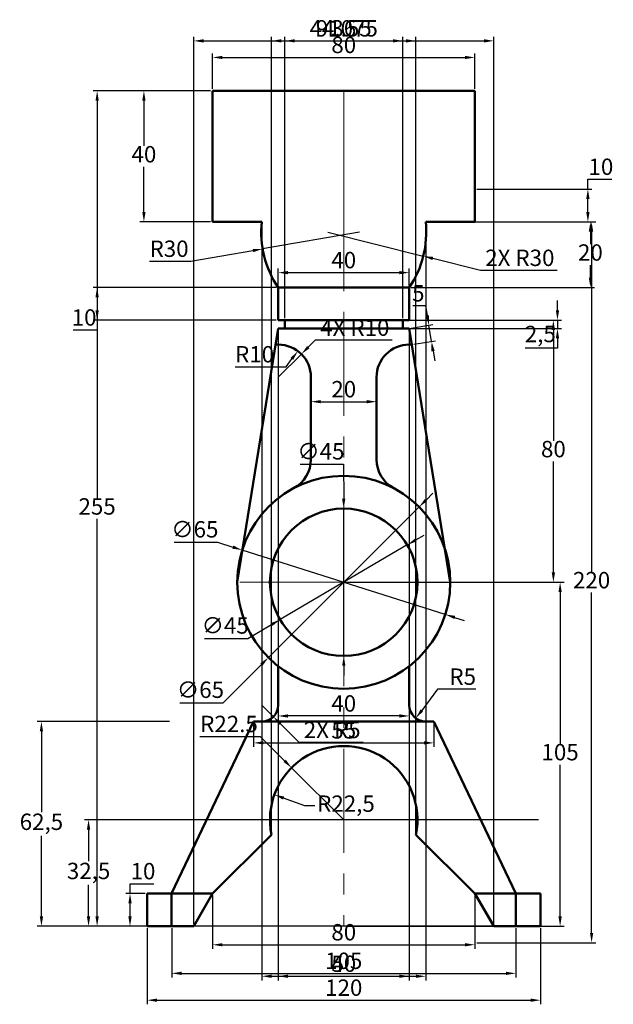
# Model space of a CAD drawing. Units: millimetres. Extents: x 61 to 242, y -47 to 253.
import ezdxf

# ---------------------------------------------------------------- set-up
doc = ezdxf.new("R2010")
doc.units = ezdxf.units.MM
doc.linetypes.add('CENTER', pattern=[50.8, 31.75, -6.35, 6.35, -6.35])
for name, color, linetype, lineweight in [('M-CNTR', 1, 'CENTER', 18), ('M-DIMS', 2, 'Continuous', 25), ('M-OUTL', 7, 'Continuous', 50)]:
    doc.layers.add(name, color=color, linetype=linetype, lineweight=lineweight)
doc.styles.get("Standard").update_dxf_attribs({"font": 'arial.ttf'})
doc.dimstyles.new('ISO-25', dxfattribs={"dimtxt": 5, "dimasz": 3, "dimexe": 1.25, "dimexo": 0.625, "dimtad": 1, "dimtih": 1, "dimtoh": 1, "dimtxsty": 'Standard', "dimcen": 2.5, "dimadec": 0, "dimazin": 0, "dimtfac": 1, "dimtmove": 0, "dimatfit": 3, "dimfxl": 1, "dimarcsym": 0})

# ---------------------------------------------------------------- blocks, each defined once
blk = doc.blocks.new('*D1')
at = {"layer": 'Defpoints', "color": 0, "transparency": 16777216}
for p in [(120.12, 231.51), (99.15, 191.51), (120.12, 191.51)]:
    blk.add_point(p, dxfattribs=at)
at = {"layer": 'M-DIMS', "color": 0, "lineweight": -2, "transparency": 16777216}
for p, q in [((119.49, 231.51), (97.9, 231.51)), ((99.15, 228.51), (99.15, 214.69)), ((99.15, 194.51), (99.15, 208.34)), ((119.49, 191.51), (97.9, 191.51))]:
    blk.add_line(p, q, dxfattribs=at)
at = {"layer": 'M-DIMS', "color": 0, "transparency": 16777216}
for points in [[(98.65, 228.51), (99.65, 228.51), (99.15, 231.51)], [(98.65, 194.51), (99.65, 194.51), (99.15, 191.51)]]:
    blk.add_solid(points, dxfattribs=at)
at = {"layer": 'M-DIMS', "color": 0, "transparency": 16777216, "insert": (99.15, 211.51), "char_height": 5, "attachment_point": 5}
blk.add_mtext('40', dxfattribs=at)
blk = doc.blocks.new('*D2')
at = {"layer": 'Defpoints', "color": 0, "transparency": 16777216}
for p in [(200.12, 241.7), (120.12, 231.51), (200.12, 231.51)]:
    blk.add_point(p, dxfattribs=at)
at = {"layer": 'M-DIMS', "color": 0, "lineweight": -2, "transparency": 16777216}
for p, q in [((120.12, 232.14), (120.12, 242.95)), ((123.12, 241.7), (197.12, 241.7)), ((200.12, 232.14), (200.12, 242.95))]:
    blk.add_line(p, q, dxfattribs=at)
at = {"layer": 'M-DIMS', "color": 0, "transparency": 16777216}
for points in [[(123.12, 242.2), (123.12, 241.2), (120.12, 241.7)], [(197.12, 242.2), (197.12, 241.2), (200.12, 241.7)]]:
    blk.add_solid(points, dxfattribs=at)
at = {"layer": 'M-DIMS', "color": 0, "transparency": 16777216, "insert": (160.12, 244.88), "char_height": 5, "attachment_point": 5}
blk.add_mtext('80', dxfattribs=at)
blk = doc.blocks.new('*D3')
at = {"layer": 'Defpoints', "color": 0, "transparency": 16777216}
for p in [(200.12, 201.51), (234.61, 201.51), (200.12, 191.51)]:
    blk.add_point(p, dxfattribs=at)
at = {"layer": 'M-DIMS', "color": 0, "lineweight": -2, "transparency": 16777216}
for p, q in [((234.61, 201.51), (234.61, 204.51)), ((234.61, 204.51), (241.91, 204.51)), ((200.74, 201.51), (235.86, 201.51)), ((234.61, 194.51), (234.61, 198.51)), ((200.74, 191.51), (235.86, 191.51))]:
    blk.add_line(p, q, dxfattribs=at)
at = {"layer": 'M-DIMS', "color": 0, "transparency": 16777216}
for points in [[(234.11, 198.51), (235.11, 198.51), (234.61, 201.51)], [(234.11, 194.51), (235.11, 194.51), (234.61, 191.51)]]:
    blk.add_solid(points, dxfattribs=at)
at = {"layer": 'M-DIMS', "color": 0, "transparency": 16777216, "insert": (238.58, 207.69), "char_height": 5, "attachment_point": 5}
blk.add_mtext('10', dxfattribs=at)
blk = doc.blocks.new('*D4')
at = {"layer": 'Defpoints', "color": 0, "transparency": 16777216}
for p in [(180.12, 176.02), (140.12, 171.51), (180.12, 171.51)]:
    blk.add_point(p, dxfattribs=at)
at = {"layer": 'M-DIMS', "color": 0, "lineweight": -2, "transparency": 16777216}
for p, q in [((140.12, 172.14), (140.12, 177.27)), ((143.12, 176.02), (177.12, 176.02)), ((180.12, 172.14), (180.12, 177.27))]:
    blk.add_line(p, q, dxfattribs=at)
at = {"layer": 'M-DIMS', "color": 0, "transparency": 16777216}
for points in [[(143.12, 176.52), (143.12, 175.52), (140.12, 176.02)], [(177.12, 176.52), (177.12, 175.52), (180.12, 176.02)]]:
    blk.add_solid(points, dxfattribs=at)
at = {"layer": 'M-DIMS', "color": 0, "transparency": 16777216, "insert": (160.12, 179.2), "char_height": 5, "attachment_point": 5}
blk.add_mtext('40', dxfattribs=at)
blk = doc.blocks.new('*D5')
at = {"layer": 'Defpoints', "color": 0, "transparency": 16777216}
for p in [(164.95, 188.35), (135.38, 183.27)]:
    blk.add_point(p, dxfattribs=at)
at = {"layer": 'M-DIMS', "color": 0, "lineweight": -2, "transparency": 16777216}
for p, q in [((164.95, 188.35), (135.38, 183.27)), ((113.42, 179.49), (132.42, 182.76)), ((100.86, 179.49), (113.42, 179.49))]:
    blk.add_line(p, q, dxfattribs=at)
at = {"layer": 'M-DIMS', "color": 0, "transparency": 16777216}
blk.add_solid([(132.34, 183.25), (132.51, 182.26), (135.38, 183.27)], dxfattribs=at)
at = {"layer": 'M-DIMS', "color": 0, "transparency": 16777216, "insert": (106.83, 182.67), "char_height": 5, "attachment_point": 5}
blk.add_mtext('R30', dxfattribs=at)
blk = doc.blocks.new('*D6')
at = {"layer": 'Defpoints', "color": 0, "transparency": 16777216}
for p in [(150.12, 144.08), (170.12, 144.08), (170.12, 136.63)]:
    blk.add_point(p, dxfattribs=at)
at = {"layer": 'M-DIMS', "color": 0, "lineweight": -2, "transparency": 16777216}
for p, q in [((150.12, 143.45), (150.12, 135.38)), ((170.12, 143.45), (170.12, 135.38)), ((153.12, 136.63), (167.12, 136.63))]:
    blk.add_line(p, q, dxfattribs=at)
at = {"layer": 'M-DIMS', "color": 0, "transparency": 16777216}
for points in [[(153.12, 137.13), (153.12, 136.13), (150.12, 136.63)], [(167.12, 137.13), (167.12, 136.13), (170.12, 136.63)]]:
    blk.add_solid(points, dxfattribs=at)
at = {"layer": 'M-DIMS', "color": 0, "transparency": 16777216, "insert": (160.12, 139.8), "char_height": 5, "attachment_point": 5}
blk.add_mtext('20', dxfattribs=at)
blk = doc.blocks.new('*D7')
at = {"layer": 'Defpoints', "color": 0, "transparency": 16777216}
for p in [(146.1, 152.09), (140.12, 144.08)]:
    blk.add_point(p, dxfattribs=at)
at = {"layer": 'M-DIMS', "color": 0, "lineweight": -2, "transparency": 16777216}
for p, q in [((126.96, 147.28), (142.51, 147.28)), ((142.51, 147.28), (144.31, 149.68))]:
    blk.add_line(p, q, dxfattribs=at)
at = {"layer": 'M-DIMS', "color": 0, "transparency": 16777216}
blk.add_solid([(143.91, 149.98), (144.71, 149.38), (146.1, 152.09)], dxfattribs=at)
at = {"layer": 'M-DIMS', "color": 0, "transparency": 16777216, "insert": (132.92, 150.46), "char_height": 5, "attachment_point": 5}
blk.add_mtext('R10', dxfattribs=at)
blk = doc.blocks.new('*D8')
at = {"layer": 'Defpoints', "color": 0, "transparency": 16777216}
for p in [(129.14, 91.34), (191.1, 71.69)]:
    blk.add_point(p, dxfattribs=at)
at = {"layer": 'M-DIMS', "color": 0, "lineweight": -2, "transparency": 16777216}
for p, q in [((108.37, 93.71), (121.64, 93.71)), ((121.64, 93.71), (126.28, 92.24)), ((191.1, 71.69), (129.14, 91.34)), ((193.96, 70.78), (196.81, 69.88))]:
    blk.add_line(p, q, dxfattribs=at)
at = {"layer": 'M-DIMS', "color": 0, "transparency": 16777216}
for points in [[(126.43, 92.72), (126.12, 91.77), (129.14, 91.34)], [(194.11, 71.26), (193.8, 70.31), (191.1, 71.69)]]:
    blk.add_solid(points, dxfattribs=at)
at = {"layer": 'M-DIMS', "color": 0, "transparency": 16777216, "insert": (114.69, 97.03), "char_height": 5, "attachment_point": 5}
blk.add_mtext('∅65', dxfattribs=at)
blk = doc.blocks.new('*D9')
at = {"layer": 'Defpoints', "color": 0, "transparency": 16777216}
for p in [(179.52, 92.9), (140.71, 70.13)]:
    blk.add_point(p, dxfattribs=at)
at = {"layer": 'M-DIMS', "color": 0, "lineweight": -2, "transparency": 16777216}
for p, q in [((182.11, 94.42), (184.7, 95.93)), ((179.52, 92.9), (140.71, 70.13)), ((130.89, 64.37), (138.12, 68.61)), ((117.62, 64.37), (130.89, 64.37))]:
    blk.add_line(p, q, dxfattribs=at)
at = {"layer": 'M-DIMS', "color": 0, "transparency": 16777216}
for points in [[(181.86, 94.85), (182.36, 93.99), (179.52, 92.9)], [(137.87, 69.04), (138.37, 68.18), (140.71, 70.13)]]:
    blk.add_solid(points, dxfattribs=at)
at = {"layer": 'M-DIMS', "color": 0, "transparency": 16777216, "insert": (123.94, 67.68), "char_height": 5, "attachment_point": 5}
blk.add_mtext('∅45', dxfattribs=at)
blk = doc.blocks.new('*D10')
at = {"layer": 'Defpoints', "color": 0, "transparency": 16777216}
for p in [(138.96, 16.66), (160.12, 9.01)]:
    blk.add_point(p, dxfattribs=at)
at = {"layer": 'M-DIMS', "color": 0, "lineweight": -2, "transparency": 16777216}
for p, q in [((148.27, 13.3), (141.78, 15.64)), ((151.27, 13.3), (148.27, 13.3))]:
    blk.add_line(p, q, dxfattribs=at)
at = {"layer": 'M-DIMS', "color": 0, "transparency": 16777216}
blk.add_solid([(141.95, 16.11), (141.61, 15.17), (138.96, 16.66)], dxfattribs=at)
at = {"layer": 'M-DIMS', "color": 0, "transparency": 16777216, "insert": (160.8, 13.3), "char_height": 5, "attachment_point": 5}
blk.add_mtext('R22,5', dxfattribs=at)
blk = doc.blocks.new('*D11')
at = {"layer": 'Defpoints', "color": 0, "transparency": 16777216}
for p in [(185.12, 44.01), (182.13, 40)]:
    blk.add_point(p, dxfattribs=at)
at = {"layer": 'M-DIMS', "color": 0, "lineweight": -2, "transparency": 16777216}
for p, q in [((188.75, 48.9), (183.92, 42.41)), ((200.47, 48.9), (188.75, 48.9))]:
    blk.add_line(p, q, dxfattribs=at)
at = {"layer": 'M-DIMS', "color": 0, "transparency": 16777216}
blk.add_solid([(183.52, 42.71), (184.32, 42.11), (182.13, 40)], dxfattribs=at)
at = {"layer": 'M-DIMS', "color": 0, "transparency": 16777216, "insert": (196.42, 52.06), "char_height": 5, "attachment_point": 5}
blk.add_mtext('R5', dxfattribs=at)
blk = doc.blocks.new('*D12')
at = {"layer": 'Defpoints', "color": 0, "transparency": 16777216}
for p in [(132.62, 39.01), (187.62, 39.01), (187.62, 32.49)]:
    blk.add_point(p, dxfattribs=at)
at = {"layer": 'M-DIMS', "color": 0, "lineweight": -2, "transparency": 16777216}
for p, q in [((132.62, 38.39), (132.62, 31.24)), ((187.62, 38.39), (187.62, 31.24)), ((135.62, 32.49), (184.62, 32.49))]:
    blk.add_line(p, q, dxfattribs=at)
at = {"layer": 'M-DIMS', "color": 0, "transparency": 16777216}
for points in [[(135.62, 32.99), (135.62, 31.99), (132.62, 32.49)], [(184.62, 32.99), (184.62, 31.99), (187.62, 32.49)]]:
    blk.add_solid(points, dxfattribs=at)
at = {"layer": 'M-DIMS', "color": 0, "transparency": 16777216, "insert": (160.12, 35.66), "char_height": 5, "attachment_point": 5}
blk.add_mtext('55', dxfattribs=at)
blk = doc.blocks.new('*D13')
at = {"layer": 'Defpoints', "color": 0, "transparency": 16777216}
for p in [(140.12, 44.01), (180.12, 44.01), (140.12, 40.71)]:
    blk.add_point(p, dxfattribs=at)
at = {"layer": 'M-DIMS', "color": 0, "lineweight": -2, "transparency": 16777216}
for p, q in [((140.12, 43.39), (140.12, 39.46)), ((180.12, 43.39), (180.12, 39.46)), ((177.12, 40.71), (143.12, 40.71))]:
    blk.add_line(p, q, dxfattribs=at)
at = {"layer": 'M-DIMS', "color": 0, "transparency": 16777216}
for points in [[(143.12, 41.21), (143.12, 40.21), (140.12, 40.71)], [(177.12, 41.21), (177.12, 40.21), (180.12, 40.71)]]:
    blk.add_solid(points, dxfattribs=at)
at = {"layer": 'M-DIMS', "color": 0, "transparency": 16777216, "insert": (160.12, 43.88), "char_height": 5, "attachment_point": 5}
blk.add_mtext('40', dxfattribs=at)
blk = doc.blocks.new('*D14')
at = {"layer": 'Defpoints', "color": 0, "transparency": 16777216}
for p in [(160.12, 161.51), (224.08, 161.51), (160.12, 81.51)]:
    blk.add_point(p, dxfattribs=at)
at = {"layer": 'M-DIMS', "color": 0, "lineweight": -2, "transparency": 16777216}
for p, q in [((160.74, 161.51), (225.33, 161.51)), ((224.08, 158.51), (224.08, 124.69)), ((224.08, 84.51), (224.08, 118.34)), ((160.74, 81.51), (225.33, 81.51))]:
    blk.add_line(p, q, dxfattribs=at)
at = {"layer": 'M-DIMS', "color": 0, "transparency": 16777216}
for points in [[(223.58, 158.51), (224.58, 158.51), (224.08, 161.51)], [(223.58, 84.51), (224.58, 84.51), (224.08, 81.51)]]:
    blk.add_solid(points, dxfattribs=at)
at = {"layer": 'M-DIMS', "color": 0, "transparency": 16777216, "insert": (224.08, 121.51), "char_height": 5, "attachment_point": 5}
blk.add_mtext('80', dxfattribs=at)
blk = doc.blocks.new('*D15')
at = {"layer": 'Defpoints', "color": 0, "transparency": 16777216}
for p in [(178.12, 161.51), (178.12, 159.01), (225.33, 159.01)]:
    blk.add_point(p, dxfattribs=at)
at = {"layer": 'M-DIMS', "color": 0, "lineweight": -2, "transparency": 16777216}
for p, q in [((225.33, 164.51), (225.33, 167.51)), ((178.74, 161.51), (226.58, 161.51)), ((225.33, 161.51), (225.33, 159.01)), ((178.74, 159.01), (226.58, 159.01)), ((225.33, 156.01), (225.33, 153.01)), ((225.33, 153.01), (215.48, 153.01))]:
    blk.add_line(p, q, dxfattribs=at)
at = {"layer": 'M-DIMS', "color": 0, "transparency": 16777216}
for points in [[(224.83, 164.51), (225.83, 164.51), (225.33, 161.51)], [(224.83, 156.01), (225.83, 156.01), (225.33, 159.01)]]:
    blk.add_solid(points, dxfattribs=at)
at = {"layer": 'M-DIMS', "color": 0, "transparency": 16777216, "insert": (220.09, 156.64), "char_height": 5, "attachment_point": 5}
blk.add_mtext('2,5', dxfattribs=at)
blk = doc.blocks.new('*D16')
at = {"layer": 'Defpoints', "color": 0, "transparency": 16777216}
for p in [(186.1, 159.98), (180.12, 159.01), (180.91, 154.08)]:
    blk.add_point(p, dxfattribs=at)
at = {"layer": 'M-DIMS', "color": 0, "lineweight": -2, "transparency": 16777216}
for p, q in [((185.15, 165.9), (181.21, 165.9)), ((185.63, 162.94), (185.15, 165.9)), ((180.73, 159.11), (187.34, 160.18)), ((186.9, 155.04), (186.1, 159.98)), ((181.53, 154.18), (188.13, 155.24)), ((187.38, 152.08), (187.86, 149.12))]:
    blk.add_line(p, q, dxfattribs=at)
at = {"layer": 'M-DIMS', "color": 0, "transparency": 16777216}
for points in [[(186.12, 163.02), (185.13, 162.86), (186.1, 159.98)], [(187.87, 152.16), (186.88, 152), (186.9, 155.04)]]:
    blk.add_solid(points, dxfattribs=at)
at = {"layer": 'M-DIMS', "color": 0, "transparency": 16777216, "insert": (182.87, 169.07), "char_height": 5, "attachment_point": 5}
blk.add_mtext('5', dxfattribs=at)
blk = doc.blocks.new('*D17')
at = {"layer": 'Defpoints', "color": 0, "transparency": 16777216}
for p in [(94.91, -13.49), (100.12, -13.49), (100.12, -23.49)]:
    blk.add_point(p, dxfattribs=at)
at = {"layer": 'M-DIMS', "color": 0, "lineweight": -2, "transparency": 16777216}
for p, q in [((94.91, -13.49), (94.91, -10.49)), ((94.91, -10.49), (102.21, -10.49)), ((99.49, -13.49), (93.66, -13.49)), ((94.91, -20.49), (94.91, -16.49)), ((99.49, -23.49), (93.66, -23.49))]:
    blk.add_line(p, q, dxfattribs=at)
at = {"layer": 'M-DIMS', "color": 0, "transparency": 16777216}
for points in [[(94.41, -16.49), (95.41, -16.49), (94.91, -13.49)], [(94.41, -20.49), (95.41, -20.49), (94.91, -23.49)]]:
    blk.add_solid(points, dxfattribs=at)
at = {"layer": 'M-DIMS', "color": 0, "transparency": 16777216, "insert": (98.87, -7.31), "char_height": 5, "attachment_point": 5}
blk.add_mtext('10', dxfattribs=at)
blk = doc.blocks.new('*D18')
at = {"layer": 'Defpoints', "color": 0, "transparency": 16777216}
for p in [(120.12, -13.49), (200.12, -13.49), (200.12, -29.13)]:
    blk.add_point(p, dxfattribs=at)
at = {"layer": 'M-DIMS', "color": 0, "lineweight": -2, "transparency": 16777216}
for p, q in [((120.12, -14.11), (120.12, -30.38)), ((200.12, -14.11), (200.12, -30.38)), ((123.12, -29.13), (197.12, -29.13))]:
    blk.add_line(p, q, dxfattribs=at)
at = {"layer": 'M-DIMS', "color": 0, "transparency": 16777216}
for points in [[(123.12, -28.63), (123.12, -29.63), (120.12, -29.13)], [(197.12, -28.63), (197.12, -29.63), (200.12, -29.13)]]:
    blk.add_solid(points, dxfattribs=at)
at = {"layer": 'M-DIMS', "color": 0, "transparency": 16777216, "insert": (160.12, -25.95), "char_height": 5, "attachment_point": 5}
blk.add_mtext('80', dxfattribs=at)
blk = doc.blocks.new('*D19')
at = {"layer": 'Defpoints', "color": 0, "transparency": 16777216}
for p in [(107.62, -23.49), (212.62, -23.49), (212.62, -37.85)]:
    blk.add_point(p, dxfattribs=at)
at = {"layer": 'M-DIMS', "color": 0, "lineweight": -2, "transparency": 16777216}
for p, q in [((107.62, -24.11), (107.62, -39.1)), ((212.62, -24.11), (212.62, -39.1)), ((110.62, -37.85), (209.62, -37.85))]:
    blk.add_line(p, q, dxfattribs=at)
at = {"layer": 'M-DIMS', "color": 0, "transparency": 16777216}
for points in [[(110.62, -37.35), (110.62, -38.35), (107.62, -37.85)], [(209.62, -37.35), (209.62, -38.35), (212.62, -37.85)]]:
    blk.add_solid(points, dxfattribs=at)
at = {"layer": 'M-DIMS', "color": 0, "transparency": 16777216, "insert": (160.12, -34.67), "char_height": 5, "attachment_point": 5}
blk.add_mtext('105', dxfattribs=at)
blk = doc.blocks.new('*D20')
at = {"layer": 'Defpoints', "color": 0, "transparency": 16777216}
for p in [(100.12, -23.49), (220.12, -23.49), (220.12, -46.05)]:
    blk.add_point(p, dxfattribs=at)
at = {"layer": 'M-DIMS', "color": 0, "lineweight": -2, "transparency": 16777216}
for p, q in [((100.12, -24.11), (100.12, -47.3)), ((220.12, -24.11), (220.12, -47.3)), ((103.12, -46.05), (217.12, -46.05))]:
    blk.add_line(p, q, dxfattribs=at)
at = {"layer": 'M-DIMS', "color": 0, "transparency": 16777216}
for points in [[(103.12, -45.55), (103.12, -46.55), (100.12, -46.05)], [(217.12, -45.55), (217.12, -46.55), (220.12, -46.05)]]:
    blk.add_solid(points, dxfattribs=at)
at = {"layer": 'M-DIMS', "color": 0, "transparency": 16777216, "insert": (160.12, -42.87), "char_height": 5, "attachment_point": 5}
blk.add_mtext('120', dxfattribs=at)
blk = doc.blocks.new('*D21')
at = {"layer": 'Defpoints', "color": 0, "transparency": 16777216}
for p in [(200.12, 191.51), (200.12, -28.49), (235.74, -28.49)]:
    blk.add_point(p, dxfattribs=at)
at = {"layer": 'M-DIMS', "color": 0, "lineweight": -2, "transparency": 16777216}
for p, q in [((200.74, 191.51), (236.99, 191.51)), ((235.74, 188.51), (235.74, 84.69)), ((235.74, -25.49), (235.74, 78.34)), ((200.74, -28.49), (236.99, -28.49))]:
    blk.add_line(p, q, dxfattribs=at)
at = {"layer": 'M-DIMS', "color": 0, "transparency": 16777216}
for points in [[(235.24, 188.51), (236.24, 188.51), (235.74, 191.51)], [(235.24, -25.49), (236.24, -25.49), (235.74, -28.49)]]:
    blk.add_solid(points, dxfattribs=at)
at = {"layer": 'M-DIMS', "color": 0, "transparency": 16777216, "insert": (235.74, 81.51), "char_height": 5, "attachment_point": 5}
blk.add_mtext('220', dxfattribs=at)
blk = doc.blocks.new('*D22')
at = {"layer": 'Defpoints', "color": 0, "transparency": 16777216}
for p in [(160.12, 81.51), (160.12, -23.49), (226.13, -23.49)]:
    blk.add_point(p, dxfattribs=at)
at = {"layer": 'M-DIMS', "color": 0, "lineweight": -2, "transparency": 16777216}
for p, q in [((160.74, 81.51), (227.38, 81.51)), ((226.13, 78.51), (226.13, 32.19)), ((226.13, -20.49), (226.13, 25.84)), ((160.74, -23.49), (227.38, -23.49))]:
    blk.add_line(p, q, dxfattribs=at)
at = {"layer": 'M-DIMS', "color": 0, "transparency": 16777216}
for points in [[(225.63, 78.51), (226.63, 78.51), (226.13, 81.51)], [(225.63, -20.49), (226.63, -20.49), (226.13, -23.49)]]:
    blk.add_solid(points, dxfattribs=at)
at = {"layer": 'M-DIMS', "color": 0, "transparency": 16777216, "insert": (226.13, 29.01), "char_height": 5, "attachment_point": 5}
blk.add_mtext('105', dxfattribs=at)
blk = doc.blocks.new('*D23')
at = {"layer": 'Defpoints', "color": 0, "transparency": 16777216}
for p in [(82.26, 9.01), (220.12, 9.01), (220.12, -23.49)]:
    blk.add_point(p, dxfattribs=at)
at = {"layer": 'M-DIMS', "color": 0, "lineweight": -2, "transparency": 16777216}
for p, q in [((219.49, 9.01), (81.01, 9.01)), ((82.26, 6.01), (82.26, -3.61)), ((82.26, -20.49), (82.26, -10.87)), ((219.49, -23.49), (81.01, -23.49))]:
    blk.add_line(p, q, dxfattribs=at)
at = {"layer": 'M-DIMS', "color": 0, "transparency": 16777216}
for points in [[(81.76, 6.01), (82.76, 6.01), (82.26, 9.01)], [(81.76, -20.49), (82.76, -20.49), (82.26, -23.49)]]:
    blk.add_solid(points, dxfattribs=at)
at = {"layer": 'M-DIMS', "color": 0, "transparency": 16777216, "insert": (82.26, -7.24), "char_height": 5, "attachment_point": 5}
blk.add_mtext('32,5', dxfattribs=at)
blk = doc.blocks.new('*D24')
at = {"layer": 'Defpoints', "color": 0, "transparency": 16777216}
for p in [(67.88, 39.01), (107.62, 39.01), (107.62, -23.49)]:
    blk.add_point(p, dxfattribs=at)
at = {"layer": 'M-DIMS', "color": 0, "lineweight": -2, "transparency": 16777216}
for p, q in [((106.99, 39.01), (66.63, 39.01)), ((67.88, 36.01), (67.88, 11.39)), ((67.88, -20.49), (67.88, 4.13)), ((106.99, -23.49), (66.63, -23.49))]:
    blk.add_line(p, q, dxfattribs=at)
at = {"layer": 'M-DIMS', "color": 0, "transparency": 16777216}
for points in [[(67.38, 36.01), (68.38, 36.01), (67.88, 39.01)], [(67.38, -20.49), (68.38, -20.49), (67.88, -23.49)]]:
    blk.add_solid(points, dxfattribs=at)
at = {"layer": 'M-DIMS', "color": 0, "transparency": 16777216, "insert": (67.88, 7.76), "char_height": 5, "attachment_point": 5}
blk.add_mtext('62,5', dxfattribs=at)
blk = doc.blocks.new('*D25')
at = {"layer": 'Defpoints', "color": 0, "transparency": 16777216}
for p in [(84.87, 231.51), (120.12, 231.51), (100.12, -23.49)]:
    blk.add_point(p, dxfattribs=at)
at = {"layer": 'M-DIMS', "color": 0, "lineweight": -2, "transparency": 16777216}
for p, q in [((119.49, 231.51), (83.62, 231.51)), ((84.87, 228.51), (84.87, 107.19)), ((84.87, -20.49), (84.87, 100.84)), ((99.49, -23.49), (83.62, -23.49))]:
    blk.add_line(p, q, dxfattribs=at)
at = {"layer": 'M-DIMS', "color": 0, "transparency": 16777216}
for points in [[(84.37, 228.51), (85.37, 228.51), (84.87, 231.51)], [(84.37, -20.49), (85.37, -20.49), (84.87, -23.49)]]:
    blk.add_solid(points, dxfattribs=at)
at = {"layer": 'M-DIMS', "color": 0, "transparency": 16777216, "insert": (84.87, 104.01), "char_height": 5, "attachment_point": 5}
blk.add_mtext('255', dxfattribs=at)
blk = doc.blocks.new('*D26')
at = {"layer": 'Defpoints', "color": 0, "transparency": 16777216}
for p in [(135.12, 191.51), (185.12, 191.51), (185.12, -38.74)]:
    blk.add_point(p, dxfattribs=at)
at = {"layer": 'M-DIMS', "color": 0, "lineweight": -2, "transparency": 16777216}
for p, q in [((135.12, 190.89), (135.12, -39.99)), ((185.12, 190.89), (185.12, -39.99)), ((138.12, -38.74), (182.12, -38.74))]:
    blk.add_line(p, q, dxfattribs=at)
at = {"layer": 'M-DIMS', "color": 0, "transparency": 16777216}
for points in [[(138.12, -38.24), (138.12, -39.24), (135.12, -38.74)], [(182.12, -38.24), (182.12, -39.24), (185.12, -38.74)]]:
    blk.add_solid(points, dxfattribs=at)
at = {"layer": 'M-DIMS', "color": 0, "transparency": 16777216, "insert": (160.12, -35.56), "char_height": 5, "attachment_point": 5}
blk.add_mtext('50', dxfattribs=at)
blk = doc.blocks.new('*D27')
at = {"layer": 'Defpoints', "color": 0, "transparency": 16777216}
for p in [(140.12, 171.51), (84.87, 161.51), (140.12, 161.51)]:
    blk.add_point(p, dxfattribs=at)
at = {"layer": 'M-DIMS', "color": 0, "lineweight": -2, "transparency": 16777216}
for p, q in [((139.49, 171.51), (83.62, 171.51)), ((84.87, 168.51), (84.87, 164.51)), ((139.49, 161.51), (83.62, 161.51)), ((84.87, 161.51), (84.87, 158.51)), ((84.87, 158.51), (77.57, 158.51))]:
    blk.add_line(p, q, dxfattribs=at)
at = {"layer": 'M-DIMS', "color": 0, "transparency": 16777216}
for points in [[(84.37, 168.51), (85.37, 168.51), (84.87, 171.51)], [(84.37, 164.51), (85.37, 164.51), (84.87, 161.51)]]:
    blk.add_solid(points, dxfattribs=at)
at = {"layer": 'M-DIMS', "color": 0, "transparency": 16777216, "insert": (80.9, 161.69), "char_height": 5, "attachment_point": 5}
blk.add_mtext('10', dxfattribs=at)
blk = doc.blocks.new('*D28')
at = {"layer": 'Defpoints', "color": 0, "transparency": 16777216}
for p in [(185.12, 191.51), (180.12, 171.51), (235.37, 171.51)]:
    blk.add_point(p, dxfattribs=at)
at = {"layer": 'M-DIMS', "color": 0, "lineweight": -2, "transparency": 16777216}
for p, q in [((185.74, 191.51), (236.62, 191.51)), ((235.37, 188.51), (235.37, 184.69)), ((235.37, 174.51), (235.37, 178.34)), ((180.74, 171.51), (236.62, 171.51))]:
    blk.add_line(p, q, dxfattribs=at)
at = {"layer": 'M-DIMS', "color": 0, "transparency": 16777216}
for points in [[(234.87, 188.51), (235.87, 188.51), (235.37, 191.51)], [(234.87, 174.51), (235.87, 174.51), (235.37, 171.51)]]:
    blk.add_solid(points, dxfattribs=at)
at = {"layer": 'M-DIMS', "color": 0, "transparency": 16777216, "insert": (235.37, 181.51), "char_height": 5, "attachment_point": 5}
blk.add_mtext('20', dxfattribs=at)
blk = doc.blocks.new('*D29')
at = {"layer": 'Defpoints', "color": 0, "transparency": 16777216}
for p in [(178.12, 246.76), (142.12, 161.51), (178.12, 161.51)]:
    blk.add_point(p, dxfattribs=at)
at = {"layer": 'M-DIMS', "color": 0, "lineweight": -2, "transparency": 16777216}
for p, q in [((142.12, 162.14), (142.12, 248.01)), ((145.12, 246.76), (175.12, 246.76)), ((178.12, 162.14), (178.12, 248.01))]:
    blk.add_line(p, q, dxfattribs=at)
at = {"layer": 'M-DIMS', "color": 0, "transparency": 16777216}
for points in [[(145.12, 247.26), (145.12, 246.26), (142.12, 246.76)], [(175.12, 247.26), (175.12, 246.26), (178.12, 246.76)]]:
    blk.add_solid(points, dxfattribs=at)
at = {"layer": 'M-DIMS', "color": 0, "transparency": 16777216, "insert": (160.12, 249.94), "char_height": 5, "attachment_point": 5}
blk.add_mtext('36', dxfattribs=at)
blk = doc.blocks.new('*D30')
at = {"layer": 'Defpoints', "color": 0, "transparency": 16777216}
for p in [(140.12, 159.01), (180.12, 159.01), (180.12, -38.74)]:
    blk.add_point(p, dxfattribs=at)
at = {"layer": 'M-DIMS', "color": 0, "lineweight": -2, "transparency": 16777216}
for p, q in [((140.12, 158.39), (140.12, -39.99)), ((180.12, 158.39), (180.12, -39.99)), ((143.12, -38.74), (177.12, -38.74))]:
    blk.add_line(p, q, dxfattribs=at)
at = {"layer": 'M-DIMS', "color": 0, "transparency": 16777216}
for points in [[(143.12, -38.24), (143.12, -39.24), (140.12, -38.74)], [(177.12, -38.24), (177.12, -39.24), (180.12, -38.74)]]:
    blk.add_solid(points, dxfattribs=at)
at = {"layer": 'M-DIMS', "color": 0, "transparency": 16777216, "insert": (160.12, -35.56), "char_height": 5, "attachment_point": 5}
blk.add_mtext('40', dxfattribs=at)
blk = doc.blocks.new('*D31')
at = {"layer": 'Defpoints', "color": 0, "transparency": 16777216}
for p in [(182.15, 246.76), (138.08, 4.48), (182.15, 4.48)]:
    blk.add_point(p, dxfattribs=at)
at = {"layer": 'M-DIMS', "color": 0, "lineweight": -2, "transparency": 16777216}
for p, q in [((138.08, 5.1), (138.08, 248.01)), ((141.08, 246.76), (179.15, 246.76)), ((182.15, 5.1), (182.15, 248.01))]:
    blk.add_line(p, q, dxfattribs=at)
at = {"layer": 'M-DIMS', "color": 0, "transparency": 16777216}
for points in [[(141.08, 247.26), (141.08, 246.26), (138.08, 246.76)], [(179.15, 247.26), (179.15, 246.26), (182.15, 246.76)]]:
    blk.add_solid(points, dxfattribs=at)
at = {"layer": 'M-DIMS', "color": 0, "transparency": 16777216, "insert": (160.12, 249.94), "char_height": 5, "attachment_point": 5}
blk.add_mtext('44.075', dxfattribs=at)
blk = doc.blocks.new('*D32')
at = {"layer": 'Defpoints', "color": 0, "transparency": 16777216}
for p in [(205.89, 246.76), (114.34, -23.49), (205.89, -23.49)]:
    blk.add_point(p, dxfattribs=at)
at = {"layer": 'M-DIMS', "color": 0, "lineweight": -2, "transparency": 16777216}
for p, q in [((114.34, -22.86), (114.34, 248.01)), ((117.34, 246.76), (202.89, 246.76)), ((205.89, -22.86), (205.89, 248.01))]:
    blk.add_line(p, q, dxfattribs=at)
at = {"layer": 'M-DIMS', "color": 0, "transparency": 16777216}
for points in [[(117.34, 247.26), (117.34, 246.26), (114.34, 246.76)], [(202.89, 247.26), (202.89, 246.26), (205.89, 246.76)]]:
    blk.add_solid(points, dxfattribs=at)
at = {"layer": 'M-DIMS', "color": 0, "transparency": 16777216, "insert": (160.12, 249.94), "char_height": 5, "attachment_point": 5}
blk.add_mtext('91.55', dxfattribs=at)
blk = doc.blocks.new('*D33')
at = {"layer": 'Defpoints', "color": 0, "transparency": 16777216}
for p in [(183.1, 104.49), (137.13, 58.53)]:
    blk.add_point(p, dxfattribs=at)
at = {"layer": 'M-DIMS', "color": 0, "lineweight": -2, "transparency": 16777216}
for p, q in [((185.22, 106.61), (187.34, 108.74)), ((183.1, 104.49), (137.13, 58.53)), ((123.34, 44.75), (135.01, 56.41)), ((110.08, 44.75), (123.34, 44.75))]:
    blk.add_line(p, q, dxfattribs=at)
at = {"layer": 'M-DIMS', "color": 0, "transparency": 16777216}
for points in [[(184.87, 106.97), (185.57, 106.26), (183.1, 104.49)], [(134.66, 56.77), (135.37, 56.06), (137.13, 58.53)]]:
    blk.add_solid(points, dxfattribs=at)
at = {"layer": 'M-DIMS', "color": 0, "transparency": 16777216, "insert": (116.4, 48.06), "char_height": 5, "attachment_point": 5}
blk.add_mtext('∅65', dxfattribs=at)
blk = doc.blocks.new('*D34')
at = {"layer": 'Defpoints', "color": 0, "transparency": 16777216}
for p in [(160.1, 104.01), (160.13, 59.01)]:
    blk.add_point(p, dxfattribs=at)
at = {"layer": 'M-DIMS', "color": 0, "lineweight": -2, "transparency": 16777216}
for p, q in [((146.83, 117.51), (160.09, 117.51)), ((160.09, 117.51), (160.1, 107.01)), ((160.13, 59.01), (160.1, 104.01)), ((160.13, 56.01), (160.13, 53.01))]:
    blk.add_line(p, q, dxfattribs=at)
at = {"layer": 'M-DIMS', "color": 0, "transparency": 16777216}
for points in [[(160.6, 107.01), (159.6, 107.01), (160.1, 104.01)], [(160.63, 56.01), (159.63, 56.01), (160.13, 59.01)]]:
    blk.add_solid(points, dxfattribs=at)
at = {"layer": 'M-DIMS', "color": 0, "transparency": 16777216, "insert": (153.15, 120.83), "char_height": 5, "attachment_point": 5}
blk.add_mtext('∅45', dxfattribs=at)
blk = doc.blocks.new('*D35')
at = {"layer": 'Defpoints', "color": 0, "transparency": 16777216}
for p in [(155.28, 188.35), (184.39, 181.07)]:
    blk.add_point(p, dxfattribs=at)
at = {"layer": 'M-DIMS', "color": 0, "lineweight": -2, "transparency": 16777216}
for p, q in [((155.28, 188.35), (184.39, 181.07)), ((201.85, 176.71), (187.3, 180.34)), ((225.23, 176.71), (201.85, 176.71))]:
    blk.add_line(p, q, dxfattribs=at)
at = {"layer": 'M-DIMS', "color": 0, "transparency": 16777216}
blk.add_solid([(187.42, 180.83), (187.18, 179.86), (184.39, 181.07)], dxfattribs=at)
at = {"layer": 'M-DIMS', "color": 0, "transparency": 16777216, "insert": (213.85, 179.89), "char_height": 5, "attachment_point": 5}
blk.add_mtext('2X R30', dxfattribs=at)
blk = doc.blocks.new('*D36')
at = {"layer": 'Defpoints', "color": 0, "transparency": 16777216}
for p in [(144.19, 24.91), (160.12, 9.01)]:
    blk.add_point(p, dxfattribs=at)
at = {"layer": 'M-DIMS', "color": 0, "lineweight": -2, "transparency": 16777216}
for p, q in [((116.2, 34.45), (134.64, 34.45)), ((134.64, 34.45), (142.07, 27.03)), ((160.12, 9.01), (144.19, 24.91))]:
    blk.add_line(p, q, dxfattribs=at)
at = {"layer": 'M-DIMS', "color": 0, "transparency": 16777216}
blk.add_solid([(142.42, 27.38), (141.71, 26.67), (144.19, 24.91)], dxfattribs=at)
at = {"layer": 'M-DIMS', "color": 0, "transparency": 16777216, "insert": (125.11, 37.62), "char_height": 5, "attachment_point": 5}
blk.add_mtext('R22.5', dxfattribs=at)
blk = doc.blocks.new('*D37')
at = {"layer": 'Defpoints', "color": 0, "transparency": 16777216}
for p in [(147.19, 151.15), (140.12, 144.08)]:
    blk.add_point(p, dxfattribs=at)
at = {"layer": 'M-DIMS', "color": 0, "lineweight": -2, "transparency": 16777216}
for p, q in [((151.43, 155.39), (149.31, 153.27)), ((174.93, 155.39), (151.43, 155.39)), ((140.12, 144.08), (147.19, 151.15))]:
    blk.add_line(p, q, dxfattribs=at)
at = {"layer": 'M-DIMS', "color": 0, "transparency": 16777216}
blk.add_solid([(148.95, 153.62), (149.66, 152.92), (147.19, 151.15)], dxfattribs=at)
at = {"layer": 'M-DIMS', "color": 0, "transparency": 16777216, "insert": (163.49, 158.57), "char_height": 5, "attachment_point": 5}
blk.add_mtext('4X R10', dxfattribs=at)
blk = doc.blocks.new('*D38')
at = {"layer": 'Defpoints', "color": 0, "transparency": 16777216}
for p in [(135.12, 44.01), (138.65, 40.48)]:
    blk.add_point(p, dxfattribs=at)
at = {"layer": 'M-DIMS', "color": 0, "lineweight": -2, "transparency": 16777216}
for p, q in [((135.12, 44.01), (138.65, 40.48)), ((146.5, 32.63), (140.77, 38.36)), ((166.06, 32.63), (146.5, 32.63))]:
    blk.add_line(p, q, dxfattribs=at)
at = {"layer": 'M-DIMS', "color": 0, "transparency": 16777216}
blk.add_solid([(141.13, 38.71), (140.42, 38), (138.65, 40.48)], dxfattribs=at)
at = {"layer": 'M-DIMS', "color": 0, "transparency": 16777216, "insert": (156.59, 35.8), "char_height": 5, "attachment_point": 5}
blk.add_mtext('2X R5', dxfattribs=at)

msp = doc.modelspace()

# ---------------------------------------------------------------- linework, layer by layer
at = {"layer": 'M-CNTR'}
for p, q in [((160.1154, 171.5135), (160.1154, 231.5135)), ((160.1154, 193.8867), (160.1154, 222.2813)), ((160.1154, 171.0055), (160.1154, 193.8867)), ((160.1154, 81.5135), (160.1154, 171.0055)), ((160.1154, 81.5135), (127.6154, 81.5135)), ((160.1154, 81.5135), (160.1154, 49.0135)), ((160.1154, 81.5135), (192.6154, 81.5135)), ((160.1154, 81.5135), (160.1154, -23.4865)), ((192.6154, 81.5135), (216.1928, 81.5135))]:
    msp.add_line(p, q, dxfattribs=at)
at = {"layer": 'M-OUTL'}
for p, q in [((160.1154, 231.5135), (120.1154, 231.5135)), ((120.1154, 231.5135), (120.1154, 191.5135)), ((160.1154, 231.5135), (200.1154, 231.5135)), ((200.1154, 231.5135), (200.1154, 191.5135)), ((120.1154, 191.5135), (135.1154, 191.5135)), ((200.1154, 191.5135), (185.1154, 191.5135)), ((140.1154, 161.5135), (140.1154, 171.5135)), ((140.1154, 171.5135), (180.1154, 171.5135)), ((180.1154, 171.5135), (180.1154, 161.5135)), ((160.1154, 161.5135), (140.1154, 161.5135)), ((142.1154, 161.5135), (142.1154, 159.0135)), ((160.1154, 161.5135), (180.1154, 161.5135)), ((178.1154, 161.5135), (178.1154, 159.0135)), ((140.1154, 159.0135), (127.6154, 81.5135)), ((140.1154, 159.0135), (180.1154, 159.0135)), ((180.1154, 159.0135), (192.6154, 81.5135)), ((180.1154, 159.0135), (180.9116, 154.0773)), ((140.1154, 154.0773), (139.3193, 154.0773)), ((180.9116, 154.0773), (180.1154, 154.0773)), ((150.1154, 144.0773), (150.1154, 119.0135)), ((170.1154, 144.0773), (170.1154, 119.0135)), ((140.1154, 49.0135), (140.1154, 55.8961)), ((180.1154, 44.0135), (180.1154, 55.8961)), ((140.1154, 49.0135), (140.1154, 44.0135)), ((132.6154, 39.0135), (107.6154, -13.4865)), ((135.1154, 39.0135), (132.6154, 39.0135)), ((135.1154, 39.0135), (185.1154, 39.0135)), ((185.1154, 39.0135), (187.6154, 39.0135)), ((187.6154, 39.0135), (212.6154, -13.4865)), ((120.1154, -13.4865), (138.0777, 4.4758)), ((200.1154, -13.4865), (182.1531, 4.4758)), ((100.1154, -23.4865), (100.1154, -13.4865)), ((100.1154, -13.4865), (120.1154, -13.4865)), ((107.6154, -23.4865), (107.6154, -13.4865)), ((120.1154, -13.4865), (114.3419, -23.4865)), ((200.1154, -13.4865), (205.8889, -23.4865)), ((200.1154, -13.4865), (220.1154, -13.4865)), ((212.6154, -23.4865), (212.6154, -13.4865)), ((212.6154, -23.4865), (212.6154, -13.4865)), ((220.1154, -13.4865), (220.1154, -23.4865)), ((114.3419, -23.4865), (100.1154, -23.4865)), ((114.3419, -23.4865), (107.6154, -23.4865)), ((205.8889, -23.4865), (220.1154, -23.4865)), ((205.8889, -23.4865), (212.6154, -23.4865))]:
    msp.add_line(p, q, dxfattribs=at)
for radius in [32.5, 22.5]:
    msp.add_circle((160.1154, 81.5135), radius, dxfattribs=at)
for centre, radius, start, end in [((164.9478, 188.3466), 30, 173.940365, 214.132122), ((155.283, 188.3466), 30, 325.867878, 6.059635), ((140.1154, 144.0773), 10, 0, 90), ((180.1154, 144.0773), 10, 90, 180), ((140.1154, 119.0135), 10, 298.072487, 0), ((180.1154, 119.0135), 10, 180, 241.927513), ((135.1154, 44.0135), 5, 270, 0), ((185.1154, 44.0135), 5, 180, 270), ((160.1154, 9.0135), 22.5, 348.365088, 191.634912)]:
    msp.add_arc(centre, radius, start, end, dxfattribs=at)

# ---------------------------------------------------------------- dimensions: what is measured, and where the dimension line sits
at = {"layer": 'M-DIMS'}
for base, p1, p2, override, picture, middle in [((205.8889, 246.7635), (114.3419, -23.4865), (205.8889, -23.4865), {"dimdec": 2, "dimlfac": 1, "dimrnd": 0, "dimzin": 0, "dimdsep": 46, "dimlunit": 2}, '*D32', (160.1154, 249.9414)), ((182.1531, 246.7635), (138.0777, 4.4758), (182.1531, 4.4758), {"dimdec": 3, "dimlfac": 1, "dimrnd": 0, "dimzin": 0, "dimdsep": 46, "dimlunit": 2}, '*D31', (160.1154, 249.9414)), ((178.1154, 246.7635), (142.1154, 161.5135), (178.1154, 161.5135), {"dimdec": 0, "dimlfac": 1, "dimrnd": 0, "dimzin": 0, "dimdsep": 46, "dimlunit": 2}, '*D29', (160.1154, 249.9431)), ((200.1154, 241.7028), (120.1154, 231.5135), (200.1154, 231.5135), {"dimclrd": 0, "dimclre": 0, "dimclrt": 0}, '*D2', (160.1154, 244.8807)), ((185.1154, -38.7365), (135.1154, 191.5135), (185.1154, 191.5135), {"dimdec": 0, "dimlfac": 1, "dimrnd": 0, "dimzin": 0, "dimdsep": 46, "dimlunit": 2}, '*D26', (160.1154, -35.5586)), ((180.1154, 176.0185), (140.1154, 171.5135), (180.1154, 171.5135), {"dimclrd": 0, "dimclre": 0, "dimclrt": 0}, '*D4', (160.1154, 179.1964)), ((180.1154, -38.7365), (140.1154, 159.0135), (180.1154, 159.0135), {"dimdec": 0, "dimlfac": 1, "dimrnd": 0, "dimzin": 0, "dimdsep": 46, "dimlunit": 2}, '*D30', (160.1154, -35.5586)), ((170.1154, 136.6268), (150.1154, 144.0773), (170.1154, 144.0773), {"dimclrd": 0, "dimclre": 0, "dimclrt": 0}, '*D6', (160.1154, 139.8047)), ((140.1154, 40.7053), (180.1154, 44.0135), (140.1154, 44.0135), {"dimclrd": 0, "dimclre": 0, "dimclrt": 0}, '*D13', (160.1154, 43.8832)), ((187.6154, 32.4943), (132.6154, 39.0135), (187.6154, 39.0135), {"dimclrd": 0, "dimclre": 0, "dimclrt": 0}, '*D12', (160.1154, 35.662)), ((200.1154, -29.132), (120.1154, -13.4865), (200.1154, -13.4865), {"dimclrd": 0, "dimclre": 0, "dimclrt": 0}, '*D18', (160.1154, -25.9541)), ((220.1154, -46.0522), (100.1154, -23.4865), (220.1154, -23.4865), {"dimclrd": 0, "dimclre": 0, "dimclrt": 0}, '*D20', (160.1154, -42.8743)), ((212.6154, -37.8499), (107.6154, -23.4865), (212.6154, -23.4865), {"dimclrd": 0, "dimclre": 0, "dimclrt": 0}, '*D19', (160.1154, -34.672))]:
    dim = msp.add_linear_dim(base=base, p1=p1, p2=p2, dimstyle='ISO-25', override=override, dxfattribs=at)
    dim.commit()
    dim.dimension.update_dxf_attribs({"geometry": picture, "text_midpoint": middle})
for base, p1, p2, override, picture, middle in [((84.8654, 231.5135), (100.1154, -23.4865), (120.1154, 231.5135), {"dimdec": 0, "dimlfac": 1, "dimrnd": 0, "dimzin": 0, "dimdsep": 46, "dimlunit": 2}, '*D25', (84.8654, 104.0135)), ((99.1453, 191.5135), (120.1154, 231.5135), (120.1154, 191.5135), {"dimclrd": 0, "dimclre": 0, "dimclrt": 0}, '*D1', (99.1453, 211.5135)), ((234.614, 201.5135), (200.1154, 191.5135), (200.1154, 201.5135), {"dimclrd": 0, "dimclre": 0, "dimclrt": 0}, '*D3', (238.5763, 207.6914)), ((235.3654, 171.5135), (185.1154, 191.5135), (180.1154, 171.5135), {"dimdec": 0, "dimlfac": 1, "dimrnd": 0, "dimzin": 0, "dimdsep": 46, "dimlunit": 2}, '*D28', (235.3654, 181.5135)), ((235.7375, -28.4865), (200.1154, 191.5135), (200.1154, -28.4865), {"dimclrd": 0, "dimclre": 0, "dimclrt": 0}, '*D21', (235.7375, 81.5135)), ((84.8654, 161.5135), (140.1154, 171.5135), (140.1154, 161.5135), {"dimdec": 0, "dimlfac": 1, "dimrnd": 0, "dimzin": 0, "dimdsep": 46, "dimlunit": 2}, '*D27', (80.9031, 161.6914)), ((225.3288, 159.0135), (178.1154, 161.5135), (178.1154, 159.0135), {"dimclrd": 0, "dimclre": 0, "dimclrt": 0}, '*D15', (220.091, 156.6433)), ((224.0788, 161.5135), (160.1154, 81.5135), (160.1154, 161.5135), {"dimclrd": 0, "dimclre": 0, "dimclrt": 0}, '*D14', (224.0788, 121.5135)), ((226.1293, -23.4865), (160.1154, 81.5135), (160.1154, -23.4865), {"dimclrd": 0, "dimclre": 0, "dimclrt": 0}, '*D22', (226.1293, 29.0135)), ((67.878, 39.0135), (107.6154, -23.4865), (107.6154, 39.0135), {"dimclrd": 0, "dimclre": 0, "dimclrt": 0}, '*D24', (67.878, 7.7635)), ((82.2623, 9.0135), (220.1154, -23.4865), (220.1154, 9.0135), {"dimclrd": 0, "dimclre": 0, "dimclrt": 0}, '*D23', (82.2623, -7.2365)), ((94.9065, -13.4865), (100.1154, -23.4865), (100.1154, -13.4865), {"dimclrd": 0, "dimclre": 0, "dimclrt": 0}, '*D17', (98.8689, -7.3086))]:
    dim = msp.add_linear_dim(base=base, p1=p1, p2=p2, angle=90, dimstyle='ISO-25', override=override, dxfattribs=at)
    dim.commit()
    dim.dimension.update_dxf_attribs({"geometry": picture, "text_midpoint": middle})
for center, mpoint, override, picture, middle in [((164.9478, 188.3466), (135.3812, 183.2658), {"dimclrd": 0, "dimclre": 0, "dimclrt": 0}, '*D5', (113.4163, 179.4913)), ((140.1154, 144.0773), (146.104, 152.0858), {"dimclrd": 0, "dimclre": 0, "dimclrt": 0}, '*D7', (132.9207, 147.2807)), ((185.1154, 44.0135), (182.132, 40.0011), {"dimclrd": 0, "dimclre": 0, "dimclrt": 0}, '*D11', (196.4215, 48.8968)), ((160.1154, 9.0135), (144.1911, 24.9089), {"dimdec": 1, "dimlfac": 1, "dimrnd": 0, "dimzin": 0, "dimdsep": 46, "dimlunit": 2}, '*D36', (125.1063, 34.4462)), ((160.1154, 9.0135), (138.9562, 16.6646), {"dimclrd": 0, "dimclre": 0, "dimclrt": 0}, '*D10', (160.8028, 13.2958))]:
    dim = msp.add_radius_dim(center=center, mpoint=mpoint, dimstyle='ISO-25', override=override, dxfattribs=at)
    dim.commit()
    dim.dimension.update_dxf_attribs({"geometry": picture, "text_midpoint": middle, "dimtype": 164})
for center, mpoint, text, picture, middle in [((155.283, 188.3466), (184.3874, 181.0709), '2X <>', '*D35', (201.85, 176.7055)), ((140.1154, 144.0773), (147.1864, 151.1484), '4X <>', '*D37', (163.4916, 155.3911))]:
    dim = msp.add_radius_dim(center=center, mpoint=mpoint, text=text, dimstyle='ISO-25', override={"dimdec": 0, "dimlfac": 1, "dimrnd": 0, "dimzin": 0, "dimdsep": 46, "dimlunit": 2}, dxfattribs=at)
    dim.commit()
    dim.dimension.update_dxf_attribs({"geometry": picture, "text_midpoint": middle, "dimtype": 164})
dim = msp.add_aligned_dim(p1=(180.9116, 154.0773), p2=(180.1154, 159.0135), distance=-6.0659, dimstyle='ISO-25', override={"dimclrd": 0, "dimclre": 0, "dimclrt": 0}, dxfattribs=at)
dim.commit()
dim.dimension.update_dxf_attribs({"geometry": '*D16', "text_midpoint": (182.8659, 169.0705)})
for p1, p2, override, picture, middle in [((160.1308, 59.0135), (160.1, 104.0135), {"dimdec": 0, "dimlfac": 1, "dimrnd": 0, "dimzin": 0, "dimdsep": 46, "dimlunit": 2}, '*D34', (153.1458, 117.5135)), ((183.0974, 104.4935), (137.1335, 58.5335), {"dimdec": 0, "dimlfac": 1, "dimrnd": 0, "dimzin": 0, "dimdsep": 46, "dimlunit": 2}, '*D33', (116.3994, 44.7455)), ((191.0955, 71.6908), (129.1353, 91.3362), {"dimclrd": 0, "dimclre": 0, "dimclrt": 0}, '*D8', (114.6913, 93.7139)), ((179.5222, 92.8988), (140.7086, 70.1281), {"dimclrd": 0, "dimclre": 0, "dimclrt": 0}, '*D9', (123.9435, 64.3669))]:
    dim = msp.add_diameter_dim_2p(p1=p1, p2=p2, dimstyle='ISO-25', override=override, dxfattribs=at)
    dim.commit()
    dim.dimension.update_dxf_attribs({"geometry": picture, "text_midpoint": middle, "dimtype": 163})
dim = msp.add_radius_dim(center=(135.1154, 44.0135), mpoint=(138.651, 40.478), text='2X <>', dimstyle='ISO-25', override={"dimdec": 0, "dimlfac": 1, "dimrnd": 0, "dimzin": 0, "dimdsep": 46, "dimlunit": 2}, dxfattribs=at)
dim.commit()
dim.dimension.update_dxf_attribs({"geometry": '*D38', "text_midpoint": (156.5936, 35.803)})

doc.saveas('drawing.dxf')
